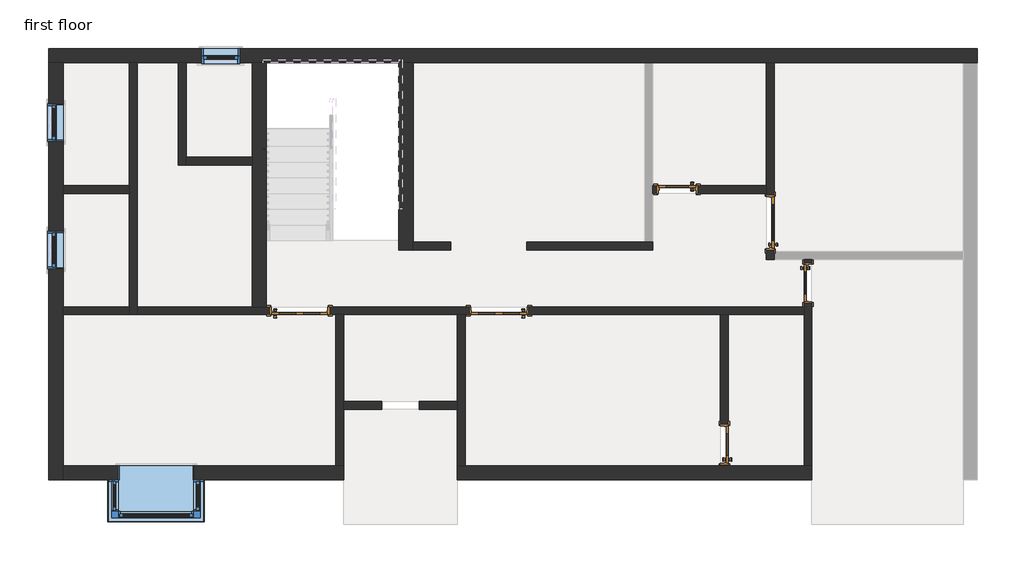
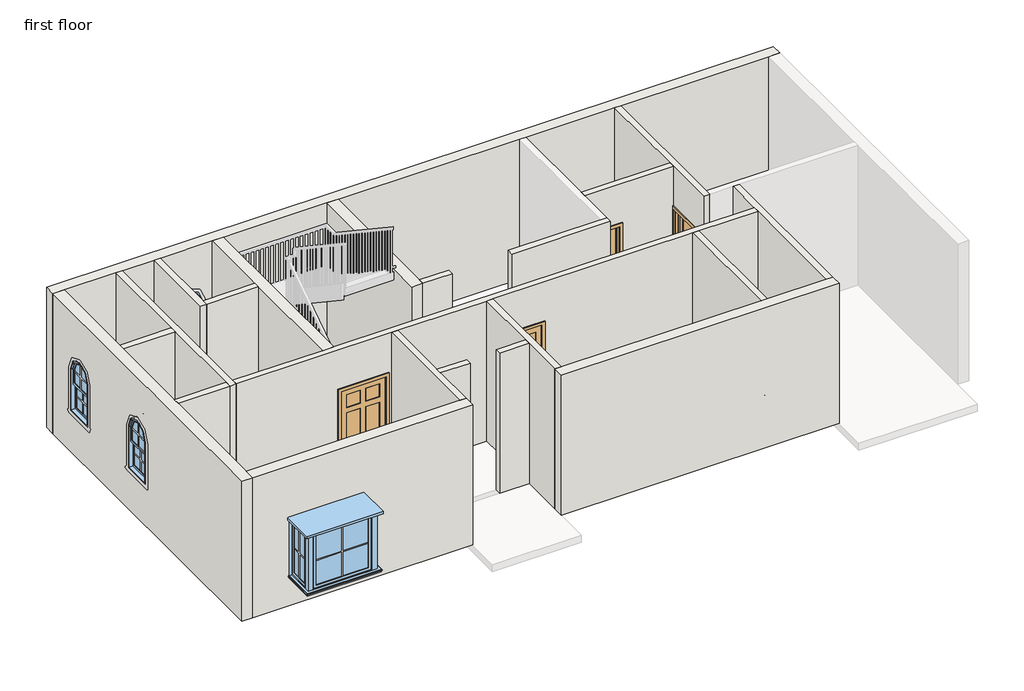
# One storey, part 1 of 3: 22 walls, 6 doors, 4 windows.
"""IFC4 building model written with IfcOpenShell, lengths in millimetres."""

from ifc_helpers import new_model, si_unit, frame, origin, place, context, project, spatial, polyline, circle_curve, outline, extrude, faceted_brep, transform, mapped, element, save
from ifc_brep_helpers import plane_surface, revolved_surface, advanced_brep
from components import door_e337afa5, door_6500584b, door_c610b25b, door_03e3dfb5, window_4fde904e, window_777a1d98

model = new_model("IFC4")

# Units and contexts
model_context = context("Model", 3, world=origin())
ifc_project = project(units=[si_unit("LENGTHUNIT", "METRE", prefix="MILLI")], contexts=[model_context])

# Site, building, storey
site = spatial("IfcSite", under=ifc_project)
building = spatial("IfcBuilding", under=site)
storey = spatial("IfcBuildingStorey", under=building, Name="first floor", Elevation=3352.8)

# Doors
placement = place(None, origin())
door_shape = door_e337afa5(model_context)
element("IfcDoor", 1, ObjectType="Door-Interior-Single-2_Panel-Wood : 24\" x 84\"", at=placement, inside=storey, context=model_context, shape_type="MappedRepresentation", body=[
    mapped(door_shape, transform((-2291.9922301, -6693.7302427, 3352.8), x_axis=(0.0, 1.0, 0.0), y_axis=(-1.0, 0.0, 0.0), z_axis=(0.0, 0.0, 1.0))),
])
element("IfcDoor", 2, ObjectType="Door-Interior-Single-2_Panel-Wood : 24\" x 84\"", at=placement, inside=storey, context=model_context, shape_type="MappedRepresentation", body=[
    mapped(door_shape, transform((-952.1422301, -4090.2302427, 3352.8), x_axis=(0.0, -1.0, 0.0), y_axis=(1.0, 0.0, 0.0), z_axis=(0.0, 0.0, 1.0))),
])
element("IfcDoor", 3, ObjectType="Door-Interior-Single-2_Panel-Wood : 24\" x 84\"", at=placement, inside=storey, context=model_context, shape_type="MappedRepresentation", body=[
    mapped(door_shape, transform((-3057.1672301, -2575.7552427, 3352.8), x_axis=(-1.0, 0.0, 0.0), y_axis=(0.0, -1.0, 0.0), z_axis=(0.0, 0.0, 1.0))),
])
door_2_shape = door_6500584b(model_context)
element("IfcDoor", 4, ObjectType="Door-Interior-Single-3_Panel_Vert-Wood : 33\" x 84\"", at=placement, inside=storey, context=model_context, shape_type="MappedRepresentation", body=[
    mapped(door_2_shape, transform((-1555.3922301, -3112.3302427, 3352.8), x_axis=(0.0, 1.0, 0.0), y_axis=(-1.0, 0.0, 0.0), z_axis=(0.0, 0.0, 1.0))),
])
door_3_shape = door_c610b25b(model_context)
element("IfcDoor", 5, ObjectType="Door-Interior-Single-6_Panel-Wood : 36\" x 84\"", at=placement, inside=storey, context=model_context, shape_type="MappedRepresentation", body=[
    mapped(door_3_shape, transform((-9140.4672301, -4537.9052427, 3352.8), x_axis=(1.0, 0.0, 0.0), y_axis=(0.0, 1.0, 0.0), z_axis=(0.0, 0.0, 1.0))),
])
door_4_shape = door_03e3dfb5(model_context)
element("IfcDoor", 6, ObjectType="Door-Interior-Single-6_Panel-Wood : 36\" x 84\"", at=placement, inside=storey, context=model_context, shape_type="MappedRepresentation", body=[
    mapped(door_4_shape, transform((-5927.3672301, -4537.9052427, 3352.8), x_axis=(-1.0, 0.0, 0.0), y_axis=(0.0, -1.0, 0.0), z_axis=(0.0, 0.0, 1.0))),
])

# Walls
element("IfcWall", 7, ObjectType="INNER WALL 5\"", at=placement, inside=storey, context=model_context, shape_type="SweptSolid", body=[
    extrude(outline(polyline([(-11883.6672301, -2642.4302427), (-12950.4672301, -2642.4302427), (-12950.4672301, -2515.4302427), (-11883.6672301, -2515.4302427), (-11883.6672301, -2642.4302427)])), frame((0.0, 0.0, 3352.8), z_axis=(0.0, 0.0, 1.0), x_axis=(1.0, 0.0, 0.0)), (0.0, 0.0, 1.0), 3048.0),
])
element("IfcWall", 8, ObjectType="INNER WALL 5\"", at=placement, inside=storey, context=model_context, shape_type="Brep", body=[
    faceted_brep([(-11883.6672301, -534.2302427, 3352.8), (-11883.6672301, -2515.4302427, 3352.8), (-11883.6672301, -2642.4302427, 3352.8), (-11883.6672301, -4471.2302427, 3352.8), (-11883.6672301, -4598.2302427, 3352.8), (-11883.6672301, -4598.2302427, 6400.8), (-11883.6672301, -4471.2302427, 6400.8), (-11883.6672301, -2642.4302427, 6400.8), (-11883.6672301, -2515.4302427, 6400.8), (-11883.6672301, -534.2302427, 6400.8), (-11756.6672301, -534.2302427, 3352.8), (-11756.6672301, -534.2302427, 6400.8), (-11756.6672301, -4471.2302427, 6400.8), (-11756.6672301, -4598.2302427, 6400.8), (-11756.6672301, -4598.2302427, 3352.8), (-11756.6672301, -4471.2302427, 3352.8)], [[[0, 1, 2, 3, 4, 5, 6, 7, 8, 9]], [[10, 11, 12, 13, 14, 15]], [[4, 3, 2, 1, 0, 10, 15, 14]], [[9, 8, 7, 6, 5, 13, 12, 11]], [[5, 4, 14, 13]], [[0, 9, 11, 10]]]),
])
element("IfcWall", 9, ObjectType="INNER WALL 5\"", at=placement, inside=storey, context=model_context, shape_type="SweptSolid", body=[
    extrude(outline(polyline([(-11883.6672301, -4598.2302427), (-12950.4672301, -4598.2302427), (-12950.4672301, -4471.2302427), (-11883.6672301, -4471.2302427), (-11883.6672301, -4598.2302427)])), frame((0.0, 0.0, 3352.8), z_axis=(0.0, 0.0, 1.0), x_axis=(1.0, 0.0, 0.0)), (0.0, 0.0, 1.0), 3048.0),
])
element("IfcWall", 10, ObjectType="INNER WALL 5\"", at=placement, inside=storey, context=model_context, shape_type="Brep", body=[
    faceted_brep([(-11096.2672301, -534.2302427, 3352.8), (-11096.2672301, -2185.2302427, 3352.8), (-11096.2672301, -2185.2302427, 6400.8), (-11096.2672301, -534.2302427, 6400.8), (-10969.2672301, -534.2302427, 3352.8), (-10969.2672301, -534.2302427, 6400.8), (-10969.2672301, -2058.2302427, 6400.8), (-10969.2672301, -2185.2302427, 6400.8), (-10969.2672301, -2185.2302427, 3352.8), (-10969.2672301, -2058.2302427, 3352.8)], [[[0, 1, 2, 3]], [[4, 5, 6, 7, 8, 9]], [[1, 0, 4, 9, 8]], [[3, 2, 7, 6, 5]], [[0, 3, 5, 4]], [[2, 1, 8, 7]]]),
])
element("IfcWall", 11, ObjectType="INNER WALL 5\"", at=placement, inside=storey, context=model_context, shape_type="SweptSolid", body=[
    extrude(outline(polyline([(-10969.2672301, -2058.2302427), (-9902.4672301, -2058.2302427), (-9902.4672301, -2185.2302427), (-10969.2672301, -2185.2302427), (-10969.2672301, -2058.2302427)])), frame((0.0, 0.0, 3352.8), z_axis=(0.0, 0.0, 1.0), x_axis=(1.0, 0.0, 0.0)), (0.0, 0.0, 1.0), 3048.0),
])
element("IfcWall", 12, ObjectType="INNER WALL 5\"", at=placement, inside=storey, context=model_context, shape_type="SweptSolid", body=[
    extrude(outline(polyline([(-6702.0672301, -3556.8302427), (-7311.6672301, -3556.8302427), (-7311.6672301, -3429.8302427), (-6702.0672301, -3429.8302427), (-6702.0672301, -3556.8302427)])), frame((0.0, 0.0, 3352.8), z_axis=(0.0, 0.0, 1.0), x_axis=(1.0, 0.0, 0.0)), (0.0, 0.0, 1.0), 3048.0),
])
element("IfcWall", 13, ObjectType="INNER WALL 5\"", at=placement, inside=storey, context=model_context, shape_type="Brep", body=[
    faceted_brep([(-5482.8672301, -3556.8302427, 3352.8), (-3450.8672301, -3556.8302427, 3352.8), (-3450.8672301, -3556.8302427, 6400.8), (-5482.8672301, -3556.8302427, 6400.8), (-5482.8672301, -3429.8302427, 3352.8), (-5482.8672301, -3429.8302427, 6400.8), (-3577.8672301, -3429.8302427, 6400.8), (-3450.8672301, -3429.8302427, 6400.8), (-3450.8672301, -3429.8302427, 3352.8), (-3577.8672301, -3429.8302427, 3352.8)], [[[0, 1, 2, 3]], [[4, 5, 6, 7, 8, 9]], [[1, 0, 4, 9, 8]], [[3, 2, 7, 6, 5]], [[0, 3, 5, 4]], [[2, 1, 8, 7]]]),
])
element("IfcWall", 14, ObjectType="INNER WALL 5\"", at=placement, inside=storey, context=model_context, shape_type="Brep", body=[
    faceted_brep([(-1622.0672301, -3709.2302427, 6400.8), (-1622.0672301, -2642.4302427, 6400.8), (-1622.0672301, -2515.4302427, 6400.8), (-1622.0672301, -534.2302427, 6400.8), (-1622.0672301, -534.2302427, 3352.8), (-1622.0672301, -2515.4302427, 3352.8), (-1622.0672301, -2642.4302427, 3352.8), (-1622.0672301, -2667.8302427, 3352.8), (-1622.0672301, -2667.8302427, 5511.8), (-1622.0672301, -3556.8302427, 5511.8), (-1622.0672301, -3556.8302427, 3352.8), (-1622.0672301, -3709.2302427, 3352.8), (-1495.0672301, -534.2302427, 6400.8), (-1495.0672301, -3582.2302427, 6400.8), (-1495.0672301, -3709.2302427, 6400.8), (-1495.0672301, -3709.2302427, 3352.8), (-1495.0672301, -3582.2302427, 3352.8), (-1495.0672301, -3556.8302427, 3352.8), (-1495.0672301, -3556.8302427, 5511.8), (-1495.0672301, -2667.8302427, 5511.8), (-1495.0672301, -2667.8302427, 3352.8), (-1495.0672301, -534.2302427, 3352.8)], [[[0, 1, 2, 3, 4, 5, 6, 7, 8, 9, 10, 11]], [[12, 13, 14, 15, 16, 17, 18, 19, 20, 21]], [[4, 21, 20, 7, 6, 5]], [[15, 11, 10, 17, 16]], [[3, 2, 1, 0, 14, 13, 12]], [[4, 3, 12, 21]], [[0, 11, 15, 14]], [[19, 8, 7, 20]], [[8, 19, 18, 9]], [[9, 18, 17, 10]]]),
])
element("IfcWall", 15, ObjectType="INNER WALL 5\"", at=placement, inside=storey, context=model_context, shape_type="SweptSolid", body=[
    extrude(outline(polyline([(6400.8, -1622.0672301), (6400.8, -3450.8672301), (3352.8, -3450.8672301), (3352.8, -3387.3672301), (5511.8, -3387.3672301), (5511.8, -2726.9672301), (3352.8, -2726.9672301), (3352.8, -1622.0672301), (6400.8, -1622.0672301)])), frame((0.0, -2642.4302427, 0.0), z_axis=(0.0, 1.0, 0.0), x_axis=(0.0, 0.0, 1.0)), (0.0, 0.0, 1.0), 127.0),
])
element("IfcWall", 16, ObjectType="INNER WALL 5\"", at=placement, inside=storey, context=model_context, shape_type="Brep", body=[
    faceted_brep([(-885.4672301, -3709.2302427, 6400.8), (-885.4672301, -7036.6302427, 6400.8), (-885.4672301, -7036.6302427, 3352.8), (-885.4672301, -4420.4302427, 3352.8), (-885.4672301, -4420.4302427, 5511.8), (-885.4672301, -3760.0302427, 5511.8), (-885.4672301, -3760.0302427, 3352.8), (-885.4672301, -3709.2302427, 3352.8), (-1012.4672301, -7036.6302427, 6400.8), (-1012.4672301, -4598.2302427, 6400.8), (-1012.4672301, -4471.2302427, 6400.8), (-1012.4672301, -3709.2302427, 6400.8), (-1012.4672301, -3709.2302427, 3352.8), (-1012.4672301, -3760.0302427, 3352.8), (-1012.4672301, -3760.0302427, 5511.8), (-1012.4672301, -4420.4302427, 5511.8), (-1012.4672301, -4420.4302427, 3352.8), (-1012.4672301, -4471.2302427, 3352.8), (-1012.4672301, -4598.2302427, 3352.8), (-1012.4672301, -7036.6302427, 3352.8)], [[[0, 1, 2, 3, 4, 5, 6, 7]], [[8, 9, 10, 11, 12, 13, 14, 15, 16, 17, 18, 19]], [[2, 19, 18, 17, 16, 3]], [[12, 7, 6, 13]], [[1, 0, 11, 10, 9, 8]], [[2, 1, 8, 19]], [[0, 7, 12, 11]], [[15, 4, 3, 16]], [[4, 15, 14, 5]], [[5, 14, 13, 6]]]),
])
element("IfcWall", 17, ObjectType="INNER WALL 5\"", at=placement, inside=storey, context=model_context, shape_type="Brep", body=[
    faceted_brep([(-11756.6672301, -4471.2302427, 6400.8), (-9902.4672301, -4471.2302427, 6400.8), (-9673.8672301, -4471.2302427, 6400.8), (-1012.4672301, -4471.2302427, 6400.8), (-1012.4672301, -4471.2302427, 3352.8), (-5444.7672301, -4471.2302427, 3352.8), (-5444.7672301, -4471.2302427, 5511.8), (-6409.9672301, -4471.2302427, 5511.8), (-6409.9672301, -4471.2302427, 3352.8), (-8657.8672301, -4471.2302427, 3352.8), (-8657.8672301, -4471.2302427, 5511.8), (-9623.0672301, -4471.2302427, 5511.8), (-9623.0672301, -4471.2302427, 3352.8), (-9673.8672301, -4471.2302427, 3352.8), (-9902.4672301, -4471.2302427, 3352.8), (-11756.6672301, -4471.2302427, 3352.8), (-1012.4672301, -4598.2302427, 6400.8), (-2231.6672301, -4598.2302427, 6400.8), (-2358.6672301, -4598.2302427, 6400.8), (-6473.4672301, -4598.2302427, 6400.8), (-6600.4672301, -4598.2302427, 6400.8), (-8429.2672301, -4598.2302427, 6400.8), (-8556.2672301, -4598.2302427, 6400.8), (-11756.6672301, -4598.2302427, 6400.8), (-11756.6672301, -4598.2302427, 3352.8), (-9623.0672301, -4598.2302427, 3352.8), (-9623.0672301, -4598.2302427, 5511.8), (-8657.8672301, -4598.2302427, 5511.8), (-8657.8672301, -4598.2302427, 3352.8), (-8556.2672301, -4598.2302427, 3352.8), (-8429.2672301, -4598.2302427, 3352.8), (-6600.4672301, -4598.2302427, 3352.8), (-6473.4672301, -4598.2302427, 3352.8), (-6409.9672301, -4598.2302427, 3352.8), (-6409.9672301, -4598.2302427, 5511.8), (-5444.7672301, -4598.2302427, 5511.8), (-5444.7672301, -4598.2302427, 3352.8), (-2358.6672301, -4598.2302427, 3352.8), (-2231.6672301, -4598.2302427, 3352.8), (-1012.4672301, -4598.2302427, 3352.8)], [[[0, 1, 2, 3, 4, 5, 6, 7, 8, 9, 10, 11, 12, 13, 14, 15]], [[16, 17, 18, 19, 20, 21, 22, 23, 24, 25, 26, 27, 28, 29, 30, 31, 32, 33, 34, 35, 36, 37, 38, 39]], [[4, 39, 38, 37, 36, 5]], [[24, 15, 14, 13, 12, 25]], [[28, 9, 8, 33, 32, 31, 30, 29]], [[3, 2, 1, 0, 23, 22, 21, 20, 19, 18, 17, 16]], [[4, 3, 16, 39]], [[0, 15, 24, 23]], [[27, 10, 9, 28]], [[10, 27, 26, 11]], [[11, 26, 25, 12]], [[7, 34, 33, 8]], [[34, 7, 6, 35]], [[35, 6, 5, 36]]]),
])
element("IfcWall", 18, ObjectType="INNER WALL 5\"", at=placement, inside=storey, context=model_context, shape_type="Brep", body=[
    faceted_brep([(-8556.2672301, -4598.2302427, 3352.8), (-8556.2672301, -7036.6302427, 3352.8), (-8556.2672301, -7036.6302427, 6400.8), (-8556.2672301, -4598.2302427, 6400.8), (-8429.2672301, -4598.2302427, 3352.8), (-8429.2672301, -4598.2302427, 6400.8), (-8429.2672301, -5995.2302427, 6400.8), (-8429.2672301, -6122.2302427, 6400.8), (-8429.2672301, -7036.6302427, 6400.8), (-8429.2672301, -7036.6302427, 3352.8), (-8429.2672301, -6122.2302427, 3352.8), (-8429.2672301, -5995.2302427, 3352.8)], [[[0, 1, 2, 3]], [[4, 5, 6, 7, 8, 9, 10, 11]], [[1, 0, 4, 11, 10, 9]], [[3, 2, 8, 7, 6, 5]], [[0, 3, 5, 4]], [[2, 1, 9, 8]]]),
])
element("IfcWall", 19, ObjectType="INNER WALL 5\"", at=placement, inside=storey, context=model_context, shape_type="SweptSolid", body=[
    extrude(outline(polyline([(-7819.6672301, -6122.2302427), (-8429.2672301, -6122.2302427), (-8429.2672301, -5995.2302427), (-7819.6672301, -5995.2302427), (-7819.6672301, -6122.2302427)])), frame((0.0, 0.0, 3352.8), z_axis=(0.0, 0.0, 1.0), x_axis=(1.0, 0.0, 0.0)), (0.0, 0.0, 1.0), 3048.0),
])
element("IfcWall", 20, ObjectType="INNER WALL 5\"", at=placement, inside=storey, context=model_context, shape_type="SweptSolid", body=[
    extrude(outline(polyline([(-6600.4672301, -6122.2302427), (-7210.0672301, -6122.2302427), (-7210.0672301, -5995.2302427), (-6600.4672301, -5995.2302427), (-6600.4672301, -6122.2302427)])), frame((0.0, 0.0, 3352.8), z_axis=(0.0, 0.0, 1.0), x_axis=(1.0, 0.0, 0.0)), (0.0, 0.0, 1.0), 3048.0),
])
element("IfcWall", 21, ObjectType="INNER WALL 5\"", at=placement, inside=storey, context=model_context, shape_type="Brep", body=[
    faceted_brep([(-6600.4672301, -4598.2302427, 3352.8), (-6600.4672301, -5995.2302427, 3352.8), (-6600.4672301, -6122.2302427, 3352.8), (-6600.4672301, -7036.6302427, 3352.8), (-6600.4672301, -7036.6302427, 6400.8), (-6600.4672301, -6122.2302427, 6400.8), (-6600.4672301, -5995.2302427, 6400.8), (-6600.4672301, -4598.2302427, 6400.8), (-6473.4672301, -4598.2302427, 3352.8), (-6473.4672301, -4598.2302427, 6400.8), (-6473.4672301, -7036.6302427, 6400.8), (-6473.4672301, -7036.6302427, 3352.8)], [[[0, 1, 2, 3, 4, 5, 6, 7]], [[8, 9, 10, 11]], [[3, 2, 1, 0, 8, 11]], [[7, 6, 5, 4, 10, 9]], [[4, 3, 11, 10]], [[0, 7, 9, 8]]]),
])
element("IfcWall", 22, ObjectType="INNER WALL 5\"", at=placement, inside=storey, context=model_context, shape_type="SweptSolid", body=[
    extrude(outline(polyline([(-7036.6302427, 6400.8), (-4598.2302427, 6400.8), (-4598.2302427, 3352.8), (-6363.5302427, 3352.8), (-6363.5302427, 5511.8), (-7023.9302427, 5511.8), (-7023.9302427, 3352.8), (-7036.6302427, 3352.8), (-7036.6302427, 6400.8)])), frame((-2358.6672301, 0.0, 0.0), z_axis=(1.0, 0.0, 0.0), x_axis=(0.0, 1.0, 0.0)), (0.0, 0.0, 1.0), 127.0),
])
element("IfcWall", 23, ObjectType="OUTER WALL 9\"", at=placement, inside=storey, context=model_context, shape_type="AdvancedBrep", body=[
    advanced_brep(
    [(-13179.0672301, -534.2302427, 3352.8), (-12950.4672301, -534.2302427, 3352.8), (-11883.6672301, -534.2302427, 3352.8), (-11756.6672301, -534.2302427, 3352.8), (-11096.2672301, -534.2302427, 3352.8), (-10969.2672301, -534.2302427, 3352.8), (-9902.4672301, -534.2302427, 3352.8), (-9673.8672301, -534.2302427, 3352.8), (-7540.2672301, -534.2302427, 3352.8), (-7311.6672301, -534.2302427, 3352.8), (-3577.8672301, -534.2302427, 3352.8), (-3450.8672301, -534.2302427, 3352.8), (-1622.0672301, -534.2302427, 3352.8), (-1495.0672301, -534.2302427, 3352.8), (1552.9327699, -534.2302427, 3352.8), (1781.5327699, -534.2302427, 3352.8), (1781.5327699, -534.2302427, 6400.8), (1552.9327699, -534.2302427, 6400.8), (-1495.0672301, -534.2302427, 6400.8), (-1622.0672301, -534.2302427, 6400.8), (-3450.8672301, -534.2302427, 6400.8), (-3577.8672301, -534.2302427, 6400.8), (-7311.6672301, -534.2302427, 6400.8), (-7540.2672301, -534.2302427, 6400.8), (-9673.8672301, -534.2302427, 6400.8), (-9902.4672301, -534.2302427, 6400.8), (-10969.2672301, -534.2302427, 6400.8), (-11096.2672301, -534.2302427, 6400.8), (-11756.6672301, -534.2302427, 6400.8), (-11883.6672301, -534.2302427, 6400.8), (-12950.4672301, -534.2302427, 6400.8), (-13179.0672301, -534.2302427, 6400.8), (-10715.2672301, -534.2302427, 5181.6), (-10105.6672301, -534.2302427, 5181.6), (-10105.6672301, -534.2302427, 4267.2), (-10715.2672301, -534.2302427, 4267.2), (-13179.0672301, -305.6302427, 3352.8), (-13179.0672301, -305.6302427, 6400.8), (1781.5327699, -305.6302427, 6400.8), (1781.5327699, -305.6302427, 3352.8), (-10715.2672301, -305.6302427, 5181.6), (-10715.2672301, -305.6302427, 4267.2), (-10105.6672301, -305.6302427, 4267.2), (-10105.6672301, -305.6302427, 5181.6)],
    [
        (0, 1),
        (1, 2),
        (2, 3),
        (3, 4),
        (4, 5),
        (5, 6),
        (6, 7),
        (7, 8),
        (8, 9),
        (9, 10),
        (10, 11),
        (11, 12),
        (12, 13),
        (13, 14),
        (14, 15),
        (15, 16),
        (16, 17),
        (17, 18),
        (18, 19),
        (19, 20),
        (20, 21),
        (21, 22),
        (22, 23),
        (23, 24),
        (24, 25),
        (25, 26),
        (26, 27),
        (27, 28),
        (28, 29),
        (29, 30),
        (30, 31),
        (31, 0),
        (32, 33, circle_curve(frame((-10410.4672301, -534.2302427, 5181.6), z_axis=(0.0, 1.0, 0.0), x_axis=(-1.0, 0.0, 0.0)), 304.8)),
        (33, 34),
        (34, 35),
        (35, 32),
        (36, 37),
        (37, 38),
        (38, 39),
        (39, 36),
        (40, 41),
        (41, 42),
        (42, 43),
        (43, 40, circle_curve(frame((-10410.4672301, -305.6302427, 5181.6), z_axis=(0.0, -1.0, 0.0), x_axis=(-1.0, 0.0, 0.0)), 304.8)),
        (0, 36),
        (39, 15),
        (16, 38),
        (37, 31),
        (32, 40),
        (43, 33),
        (42, 34),
        (41, 35),
    ],
    [
        plane_surface(frame((-13170.1356678, -534.2302427, 3352.8), z_axis=(0.0, -1.0, 0.0), x_axis=(1.0, 0.0, 0.0))),
        plane_surface(frame((-13170.1356678, -305.6302427, 3352.8), z_axis=(0.0, 1.0, 0.0), x_axis=(-1.0, 0.0, 0.0))),
        plane_surface(frame((-13064.7672301, -534.2302427, 3352.8), z_axis=(0.0, 0.0, -1.0), x_axis=(0.0, 1.0, 0.0))),
        plane_surface(frame((1667.2327699, -534.2302427, 6400.8), z_axis=(0.0, 0.0, 1.0), x_axis=(0.0, 1.0, 0.0))),
        plane_surface(frame((-13179.0672301, -534.2302427, 3352.8), z_axis=(-1.0, 0.0, 0.0), x_axis=(0.0, -1.0, 0.0))),
        plane_surface(frame((1781.5327699, -7258.6414899, 3352.8), z_axis=(1.0, 0.0, 0.0), x_axis=(0.0, 1.0, 0.0))),
        revolved_surface(polyline([(-10715.267230099998, -305.6302427, 5181.6), (-10715.267230099998, -534.2302427, 5181.6)]), (-10410.4672301, -305.6302427, 5181.6), (0.0, 1.0, 0.0)),
        plane_surface(frame((-10105.6672301, -534.2302427, 5181.6), z_axis=(-1.0, 0.0, 0.0), x_axis=(0.0, 1.0, 0.0))),
        plane_surface(frame((-10105.6672301, -534.2302427, 4267.2), z_axis=(0.0, 0.0, 1.0), x_axis=(0.0, 1.0, 0.0))),
        plane_surface(frame((-10715.2672301, -534.2302427, 4267.2), z_axis=(1.0, 0.0, 0.0), x_axis=(0.0, 1.0, 0.0))),
    ],
    [
        (0, [[1, 2, 3, 4, 5, 6, 7, 8, 9, 10, 11, 12, 13, 14, 15, 16, 17, 18, 19, 20, 21, 22, 23, 24, 25, 26, 27, 28, 29, 30, 31, 32], [33, 34, 35, 36]]),
        (1, [[37, 38, 39, 40], [41, 42, 43, 44]]),
        (2, [[-15, -14, -13, -12, -11, -10, -9, -8, -7, -6, -5, -4, -3, -2, -1, 45, -40, 46]]),
        (3, [[-31, -30, -29, -28, -27, -26, -25, -24, -23, -22, -21, -20, -19, -18, -17, 47, -38, 48]]),
        (4, [[-32, -48, -37, -45]]),
        (5, [[-16, -46, -39, -47]]),
        (6, [[-33, 49, -44, 50]]),
        (7, [[-34, -50, -43, 51]]),
        (8, [[-35, -51, -42, 52]]),
        (9, [[-36, -52, -41, -49]]),
    ],
),
])
element("IfcWall", 24, ObjectType="OUTER WALL 9\"", at=placement, inside=storey, context=model_context, shape_type="AdvancedBrep", body=[
    advanced_brep(
    [(-13179.0672301, -534.2302427, 3352.8), (-13179.0672301, -7265.2302427, 3352.8), (-13179.0672301, -7265.2302427, 6400.8), (-13179.0672301, -534.2302427, 6400.8), (-13179.0672301, -1194.6302427, 5181.6), (-13179.0672301, -1804.2302427, 5181.6), (-13179.0672301, -1804.2302427, 4267.2), (-13179.0672301, -1194.6302427, 4267.2), (-13179.0672301, -3252.0302427, 5181.6), (-13179.0672301, -3861.6302427, 5181.6), (-13179.0672301, -3861.6302427, 4267.2), (-13179.0672301, -3252.0302427, 4267.2), (-12950.4672301, -534.2302427, 3352.8), (-12950.4672301, -534.2302427, 6400.8), (-12950.4672301, -2515.4302427, 6400.8), (-12950.4672301, -2642.4302427, 6400.8), (-12950.4672301, -4471.2302427, 6400.8), (-12950.4672301, -4598.2302427, 6400.8), (-12950.4672301, -7036.6302427, 6400.8), (-12950.4672301, -7265.2302427, 6400.8), (-12950.4672301, -7265.2302427, 3352.8), (-12950.4672301, -7036.6302427, 3352.8), (-12950.4672301, -4598.2302427, 3352.8), (-12950.4672301, -4471.2302427, 3352.8), (-12950.4672301, -2642.4302427, 3352.8), (-12950.4672301, -2515.4302427, 3352.8), (-12950.4672301, -1194.6302427, 5181.6), (-12950.4672301, -1194.6302427, 4267.2), (-12950.4672301, -1804.2302427, 4267.2), (-12950.4672301, -1804.2302427, 5181.6), (-12950.4672301, -3252.0302427, 5181.6), (-12950.4672301, -3252.0302427, 4267.2), (-12950.4672301, -3861.6302427, 4267.2), (-12950.4672301, -3861.6302427, 5181.6)],
    [
        (0, 1),
        (1, 2),
        (2, 3),
        (3, 0),
        (4, 5, circle_curve(frame((-13179.0672301, -1499.4302427, 5181.6), z_axis=(1.0, 0.0, 0.0), x_axis=(0.0, 1.0, 0.0)), 304.8)),
        (5, 6),
        (6, 7),
        (7, 4),
        (8, 9, circle_curve(frame((-13179.0672301, -3556.8302427, 5181.6), z_axis=(1.0, 0.0, 0.0), x_axis=(0.0, 1.0, 0.0)), 304.8)),
        (9, 10),
        (10, 11),
        (11, 8),
        (12, 13),
        (13, 14),
        (14, 15),
        (15, 16),
        (16, 17),
        (17, 18),
        (18, 19),
        (19, 20),
        (20, 21),
        (21, 22),
        (22, 23),
        (23, 24),
        (24, 25),
        (25, 12),
        (26, 27),
        (27, 28),
        (28, 29),
        (29, 26, circle_curve(frame((-12950.4672301, -1499.4302427, 5181.6), z_axis=(-1.0, 0.0, 0.0), x_axis=(0.0, 1.0, 0.0)), 304.8)),
        (30, 31),
        (31, 32),
        (32, 33),
        (33, 30, circle_curve(frame((-12950.4672301, -3556.8302427, 5181.6), z_axis=(-1.0, 0.0, 0.0), x_axis=(0.0, 1.0, 0.0)), 304.8)),
        (0, 12),
        (20, 1),
        (2, 19),
        (13, 3),
        (4, 26),
        (29, 5),
        (28, 6),
        (27, 7),
        (8, 30),
        (33, 9),
        (32, 10),
        (31, 11),
    ],
    [
        plane_surface(frame((-13179.0672301, -534.2302427, 3352.8), z_axis=(-1.0, 0.0, 0.0), x_axis=(0.0, -1.0, 0.0))),
        plane_surface(frame((-12950.4672301, -534.2302427, 3352.8), z_axis=(1.0, 0.0, 0.0), x_axis=(0.0, 1.0, 0.0))),
        plane_surface(frame((-13179.0672301, -419.9302427, 3352.8), z_axis=(0.0, 0.0, -1.0), x_axis=(1.0, 0.0, 0.0))),
        plane_surface(frame((-13179.0672301, -7150.9302427, 6400.8), z_axis=(0.0, 0.0, 1.0), x_axis=(1.0, 0.0, 0.0))),
        plane_surface(frame((-13170.1356678, -534.2302427, 3352.8), z_axis=(0.0, 1.0, 0.0), x_axis=(1.0, 0.0, 0.0))),
        plane_surface(frame((-13179.0672301, -7265.2302427, 3352.8), z_axis=(0.0, -1.0, 0.0), x_axis=(1.0, 0.0, 0.0))),
        revolved_surface(polyline([(-12950.4672301, -1194.6302427, 5181.6), (-13179.0672301, -1194.6302427, 5181.6)]), (-12950.4672301, -1499.4302427, 5181.6), (1.0, 0.0, 0.0)),
        plane_surface(frame((-13179.0672301, -1804.2302427, 5181.6), z_axis=(0.0, 1.0, 0.0), x_axis=(1.0, 0.0, 0.0))),
        plane_surface(frame((-13179.0672301, -1804.2302427, 4267.2), z_axis=(0.0, 0.0, 1.0), x_axis=(1.0, 0.0, 0.0))),
        plane_surface(frame((-13179.0672301, -1194.6302427, 4267.2), z_axis=(0.0, -1.0, 0.0), x_axis=(1.0, 0.0, 0.0))),
        revolved_surface(polyline([(-12950.4672301, -3252.0302426999997, 5181.6), (-13179.0672301, -3252.0302426999997, 5181.6)]), (-12950.4672301, -3556.8302427, 5181.6), (1.0, 0.0, 0.0)),
        plane_surface(frame((-13179.0672301, -3861.6302427, 5181.6), z_axis=(0.0, 1.0, 0.0), x_axis=(1.0, 0.0, 0.0))),
        plane_surface(frame((-13179.0672301, -3861.6302427, 4267.2), z_axis=(0.0, 0.0, 1.0), x_axis=(1.0, 0.0, 0.0))),
        plane_surface(frame((-13179.0672301, -3252.0302427, 4267.2), z_axis=(0.0, -1.0, 0.0), x_axis=(1.0, 0.0, 0.0))),
    ],
    [
        (0, [[1, 2, 3, 4], [5, 6, 7, 8], [9, 10, 11, 12]]),
        (1, [[13, 14, 15, 16, 17, 18, 19, 20, 21, 22, 23, 24, 25, 26], [27, 28, 29, 30], [31, 32, 33, 34]]),
        (2, [[-1, 35, -26, -25, -24, -23, -22, -21, 36]]),
        (3, [[-3, 37, -19, -18, -17, -16, -15, -14, 38]]),
        (4, [[-4, -38, -13, -35]]),
        (5, [[-2, -36, -20, -37]]),
        (6, [[-5, 39, -30, 40]]),
        (7, [[-6, -40, -29, 41]]),
        (8, [[-7, -41, -28, 42]]),
        (9, [[-8, -42, -27, -39]]),
        (10, [[-9, 43, -34, 44]]),
        (11, [[-10, -44, -33, 45]]),
        (12, [[-11, -45, -32, 46]]),
        (13, [[-12, -46, -31, -43]]),
    ],
),
])
element("IfcWall", 25, ObjectType="OUTER WALL 9\"", at=placement, inside=storey, context=model_context, shape_type="Brep", body=[
    faceted_brep([(-12950.4672301, -7265.2302427, 3352.8), (-8429.2672301, -7265.2302427, 3352.8), (-8429.2672301, -7265.2302427, 6400.8), (-12950.4672301, -7265.2302427, 6400.8), (-12061.4672301, -7265.2302427, 5232.4), (-10842.2672301, -7265.2302427, 5232.4), (-10842.2672301, -7265.2302427, 3962.4), (-12061.4672301, -7265.2302427, 3962.4), (-12950.4672301, -7036.6302427, 3352.8), (-12950.4672301, -7036.6302427, 6400.8), (-8556.2672301, -7036.6302427, 6400.8), (-8429.2672301, -7036.6302427, 6400.8), (-8429.2672301, -7036.6302427, 3352.8), (-8556.2672301, -7036.6302427, 3352.8), (-12061.4672301, -7036.6302427, 5232.4), (-12061.4672301, -7036.6302427, 3962.4), (-10842.2672301, -7036.6302427, 3962.4), (-10842.2672301, -7036.6302427, 5232.4)], [[[0, 1, 2, 3], [4, 5, 6, 7]], [[8, 9, 10, 11, 12, 13], [14, 15, 16, 17]], [[1, 0, 8, 13, 12]], [[3, 2, 11, 10, 9]], [[0, 3, 9, 8]], [[15, 14, 4, 7]], [[16, 15, 7, 6]], [[17, 16, 6, 5]], [[14, 17, 5, 4]], [[2, 1, 12, 11]]]),
])
element("IfcWall", 26, ObjectType="OUTER WALL 9\"", at=placement, inside=storey, context=model_context, shape_type="Brep", body=[
    faceted_brep([(-7540.2672301, -534.2302427, 3352.8), (-7540.2672301, -3556.8302427, 3352.8), (-7540.2672301, -3556.8302427, 6400.8), (-7540.2672301, -534.2302427, 6400.8), (-7311.6672301, -534.2302427, 3352.8), (-7311.6672301, -534.2302427, 6400.8), (-7311.6672301, -3429.8302427, 6400.8), (-7311.6672301, -3556.8302427, 6400.8), (-7311.6672301, -3556.8302427, 3352.8), (-7311.6672301, -3429.8302427, 3352.8)], [[[0, 1, 2, 3]], [[4, 5, 6, 7, 8, 9]], [[1, 0, 4, 9, 8]], [[3, 2, 7, 6, 5]], [[0, 3, 5, 4]], [[2, 1, 8, 7]]]),
])
element("IfcWall", 27, ObjectType="OUTER WALL 9\"", at=placement, inside=storey, context=model_context, shape_type="Brep", body=[
    faceted_brep([(-9902.4672301, -534.2302427, 3352.8), (-9902.4672301, -2058.2302427, 3352.8), (-9902.4672301, -2185.2302427, 3352.8), (-9902.4672301, -4471.2302427, 3352.8), (-9902.4672301, -4471.2302427, 6400.8), (-9902.4672301, -2185.2302427, 6400.8), (-9902.4672301, -2058.2302427, 6400.8), (-9902.4672301, -534.2302427, 6400.8), (-9673.8672301, -534.2302427, 3352.8), (-9673.8672301, -534.2302427, 6400.8), (-9673.8672301, -4471.2302427, 6400.8), (-9673.8672301, -4471.2302427, 3352.8)], [[[0, 1, 2, 3, 4, 5, 6, 7]], [[8, 9, 10, 11]], [[3, 2, 1, 0, 8, 11]], [[7, 6, 5, 4, 10, 9]], [[0, 7, 9, 8]], [[4, 3, 11, 10]]]),
])
element("IfcWall", 28, ObjectType="OUTER WALL 9\"", at=placement, inside=storey, context=model_context, shape_type="Brep", body=[
    faceted_brep([(-6600.4672301, -7265.2302427, 3352.8), (-885.4672301, -7265.2302427, 3352.8), (-885.4672301, -7265.2302427, 6400.8), (-6600.4672301, -7265.2302427, 6400.8), (-6600.4672301, -7036.6302427, 3352.8), (-6600.4672301, -7036.6302427, 6400.8), (-6473.4672301, -7036.6302427, 6400.8), (-2358.6672301, -7036.6302427, 6400.8), (-2231.6672301, -7036.6302427, 6400.8), (-1012.4672301, -7036.6302427, 6400.8), (-885.4672301, -7036.6302427, 6400.8), (-885.4672301, -7036.6302427, 3352.8), (-1012.4672301, -7036.6302427, 3352.8), (-2231.6672301, -7036.6302427, 3352.8), (-2358.6672301, -7036.6302427, 3352.8), (-6473.4672301, -7036.6302427, 3352.8)], [[[0, 1, 2, 3]], [[4, 5, 6, 7, 8, 9, 10, 11, 12, 13, 14, 15]], [[1, 0, 4, 15, 14, 13, 12, 11]], [[3, 2, 10, 9, 8, 7, 6, 5]], [[2, 1, 11, 10]], [[0, 3, 5, 4]]]),
])

# Windows
window_shape = window_4fde904e(model_context)
element("IfcWindow", 29, ObjectType="Window-Bay-Casement-Box-90_Degree_Angle-Center_Fixed : 48\" x 48\" x 24\" 2", at=placement, inside=storey, context=model_context, shape_type="MappedRepresentation", body=[
    mapped(window_shape, transform((-11451.8672301, -7150.9302427, 3352.8), x_axis=(-1.0, 0.0, 0.0), y_axis=(0.0, -1.0, 0.0), z_axis=(0.0, 0.0, 1.0))),
])
window_2_shape = window_777a1d98(model_context)
element("IfcWindow", 30, ObjectType="Window-Double-Hung-Arch-Head : 24\" x 48\"", at=placement, inside=storey, context=model_context, shape_type="MappedRepresentation", body=[
    mapped(window_2_shape, transform((-13064.7672301, -1499.4302427, 3352.8), x_axis=(0.0, 1.0, 0.0), y_axis=(-1.0, 0.0, 0.0), z_axis=(0.0, 0.0, 1.0))),
])
element("IfcWindow", 31, ObjectType="Window-Double-Hung-Arch-Head : 24\" x 48\"", at=placement, inside=storey, context=model_context, shape_type="MappedRepresentation", body=[
    mapped(window_2_shape, transform((-13064.7672301, -3556.8302427, 3352.8), x_axis=(0.0, 1.0, 0.0), y_axis=(-1.0, 0.0, 0.0), z_axis=(0.0, 0.0, 1.0))),
])
element("IfcWindow", 32, ObjectType="Window-Double-Hung-Arch-Head : 24\" x 48\"", at=placement, inside=storey, context=model_context, shape_type="MappedRepresentation", body=[
    mapped(window_2_shape, transform((-10410.4672301, -419.9302427, 3352.8), x_axis=(-1.0, 0.0, 0.0), y_axis=(0.0, -1.0, 0.0), z_axis=(0.0, 0.0, 1.0))),
])

save(model, "model.ifc")

# Revit data of these elements
# Type "Door-Interior-Single-2_Panel-Wood : 24\" x 84\""
#   Type Mark = "10"
#   Assembly Code = "C1020300"
#   Analytic Construction = "Wooden"
#   Top Rail = 0' - 4 11/16"
#   Thickness = 0' - 1 3/8"
#   Thermal Resistance (R) = 2.5876 (h·ft²·°F)/BTU
#   Swing Angle [instance default] = 90.00°
#   Stiles = 0' - 4 3/4"
#   Rough Width = 2' - 2"
#   Rough Height = 7' - 1"
#   Lock Rail = 0' - 7 1/2"
#   Height = 7' - 0"
#   Width = 2' - 0"
#   Heat Transfer Coefficient (U) = 0.3865 BTU/(h·ft²·°F)
#   Bottom Rail = 0' - 9 1/8"
#   Trim Material = Cherry
#   Panel Material = Cherry
#   Frame Material = Cherry
#   Door Handle Material = Aluminum
#   Visual Light Transmittance = 0
#   Solar Heat Gain Coefficient = 0
#   Wall Closure = (empty or 0)
#   Function = (empty or 0)
# Type "Door-Interior-Single-3_Panel_Vert-Wood : 33\" x 84\""
#   Type Mark = "11"
#   Assembly Code = "C1020300"
#   Analytic Construction = "Wooden"
#   Top Rail = 0' - 4 11/16"
#   Thickness = 0' - 1 3/8"
#   Thermal Resistance (R) = 2.5876 (h·ft²·°F)/BTU
#   Swing Angle [instance default] = 90.00°
#   Stiles = 0' - 4 3/4"
#   Rough Width = 2' - 11"
#   Rough Height = 7' - 1"
#   Intermediate Rail = 0' - 4 1/2"
#   Height = 7' - 0"
#   Width = 2' - 9"
#   Heat Transfer Coefficient (U) = 0.3865 BTU/(h·ft²·°F)
#   Bottom Rail = 0' - 9 1/8"
#   Trim Material = Cherry
#   Panel Material = Cherry
#   Frame Material = Cherry
#   Door Handle Material = Aluminum
#   Visual Light Transmittance = 0
#   Solar Heat Gain Coefficient = 0
#   Wall Closure = (empty or 0)
#   Function = (empty or 0)
# Type "Door-Interior-Single-6_Panel-Wood : 36\" x 84\""
#   Type Mark = "12"
#   Assembly Code = "C1020300"
#   Analytic Construction = "Wooden"
#   Top Rail = 0' - 4 11/16"
#   Top Panel = 0' - 11"
#   Thickness = 0' - 1 3/8"
#   Thermal Resistance (R) = 2.5876 (h·ft²·°F)/BTU
#   Swing Angle [instance default] = 90.00°
#   Stiles = 0' - 4 3/4"
#   Rough Width = 3' - 2"
#   Rough Height = 7' - 1"
#   Mullion = 0' - 4 1/2"
#   Lock Rail = 0' - 7 1/2"
#   Intermediate Rail = 0' - 4 1/2"
#   Height = 7' - 0"
#   Width = 3' - 0"
#   Heat Transfer Coefficient (U) = 0.3865 BTU/(h·ft²·°F)
#   Bottom Rail = 0' - 9 1/8"
#   Trim Material = Cherry
#   Panel Material = Cherry
#   Frame Material = Cherry
#   Door Handle Material = Aluminum
#   Visual Light Transmittance = 0
#   Solar Heat Gain Coefficient = 0
#   Wall Closure = (empty or 0)
#   Function = (empty or 0)
# Type "INNER WALL 5\""
#   Assembly Code = "B2010"
#   Layers, outside or top first: 0' - 5" "WARM BEIGE COLOUR" (function 1)
# Type "OUTER WALL 9\""
#   Assembly Code = "B2010"
#   Layers, outside or top first: 0' - 9" "WARM BEIGE COLOUR" (function 1)
# Type "Window-Bay-Casement-Box-90_Degree_Angle-Center_Fixed : 48\" x 48\" x 24\" 2"
#   Type Mark = "22"
#   Fire Rating = "0.5h"
#   Assembly Code = "B2020100"
#   Analytic Construction = "1/8 in Pilkington single glazing"
#   Width = 4' - 0"
#   Wall Thickness [instance default] = 0' - 6"
#   Visual Light Transmittance = 0.9
#   Trim Width = 4' - 8"
#   Trim Height = 4' - 0"
#   Thermal Resistance (R) = 1.5394 (h·ft²·°F)/BTU
#   Solar Heat Gain Coefficient = 0.86
#   Rough Width = 4' - 0 1/2"
#   Rough Height = 4' - 0 1/2"
#   Height 1 = 4' - 2"
#   Height = 4' - 0"
#   Heat Transfer Coefficient (U) = 0.6496 BTU/(h·ft²·°F)
#   Depth = 2' - 0"
#   Default Sill Height = 2' - 0"
#   Side Muntin Visibility = yes
#   Center Muntin Visibility = yes
#   Interior Trim Visibility [instance default] = yes
#   Exterior Trim Visibility [instance default] = yes
#   Side Muntin Pattern = Muntin Pattern_2x2 : Muntin Pattern_2x2
#   Center Muntin Pattern = Muntin Pattern_2x2 : Muntin Pattern_2x2
#   Interior Trim Material = Wood - Stained
#   Exterior Trim Material = Clad - White
#   Exterior Trim = element 393412
#   Interior Trim = Trim-Window-Interior-Flat : Picture Frame
#   Interior Frame Material = Wood - Stained
#   Glass Panel Material = Glass
#   Exterior Frame Material = Clad - White
#   Wall Closure = (empty or 0)
# Type "Window-Double-Hung-Arch-Head : 24\" x 48\""
#   Type Mark = "19"
#   Fire Rating = "0.5h"
#   Construction Type Id = "DG-DR"
#   Assembly Code = "B2020100"
#   Analytic Construction = "Double glazing - domestic"
#   Wall Thickness [instance default] = 0' - 6"
#   Window Inset [instance default] = 0' - 0"
#   Visual Light Transmittance = 0.81
#   Thermal Resistance (R) = 1.8146 (h·ft²·°F)/BTU
#   Solar Heat Gain Coefficient = 0.76
#   Muntin Width = 1' - 6"
#   Muntin Height = 1' - 8 1/8"
#   Interior Wall Closure [instance default] = 0' - 1 1/2"
#   Rough Width = 2' - 0 1/2"
#   Rough Height = 4' - 0 1/2"
#   Half Width = 1' - 0"
#   Frame Extension [instance default] = 0' - 1 1/4"
#   Exterior Wall Closure [instance default] = 0' - 0 1/2"
#   Extension Jamb [instance default] = 0' - 1 1/2"
#   Heat Transfer Coefficient (U) = 0.5511 BTU/(h·ft²·°F)
#   Height = 4' - 0"
#   Width = 2' - 0"
#   Top Muntin Visibility = yes
#   Indicator Visibility [instance default] = yes
#   Extension Jamb Visibility [instance default] = yes
#   Interior Trim Visibility [instance default] = yes
#   Exterior Trim Visibility [instance default] = yes
#   Define Thermal Properties by = 1
#   Bottom Muntin Visibility = yes
#   Muntin Pattern = Muntin Pattern_2x2 : Muntin Pattern_2x2
#   Interior Trim Material = Wood - Stained
#   Interior Trim = Trim-Window-Interior-Arch-Hung : Picture Frame
#   Exterior Trim Material = Clad - White
#   Exterior Trim = Trim-Window-Exterior-Arch-Hung : with Sill
#   Glass Panel Material = Glass
#   Exterior Frame Material = Clad - White
#   Interior Frame Material = Wood - Stained
#   Wall Closure = (empty or 0)
# Elements 1, 2, 3 (IfcDoor, "Door-Interior-Single-2_Panel-Wood : 24\" x 84\"")
#   Swing Angle = 90.00°
#   Phase Created = New Construction
#   Materials on its faces: "Cherry", "Aluminum"
# Element 4 (IfcDoor, "Door-Interior-Single-3_Panel_Vert-Wood : 33\" x 84\"")
#   Swing Angle = 90.00°
#   Phase Created = New Construction
#   Materials on its faces: "Cherry", "Aluminum"
# Elements 5, 6 (IfcDoor, "Door-Interior-Single-6_Panel-Wood : 36\" x 84\"")
#   Swing Angle = 90.00°
#   Phase Created = New Construction
#   Materials on its faces: "Cherry", "Aluminum"
# Elements 7, 8, 9, 10, 11, 12, 13, 14, 15, 16, 17, 18, 19, 20, 21, 22 (IfcWall, "INNER WALL 5\"")
#   Top Offset = 0' - 0"
#   Base Offset = 0' - 0"
#   wall height = 10' - 0"
#   Phase Created = New Construction
#   Base Constraint = first floor
#   Top Constraint = TOP OF THE BUILDING
#   Materials on its faces: "WARM BEIGE COLOUR"
# Elements 23, 24, 25, 26, 27, 28 (IfcWall, "OUTER WALL 9\"")
#   Top Offset = 0' - 0"
#   Base Offset = 0' - 0"
#   wall height = 10' - 0"
#   Phase Created = New Construction
#   Base Constraint = first floor
#   Top Constraint = TOP OF THE BUILDING
#   Materials on its faces: "WARM BEIGE COLOUR"
# Element 29 (IfcWindow, "Window-Bay-Casement-Box-90_Degree_Angle-Center_Fixed : 48\" x 48\" x 24\" 2")
#   Mark = "8"
#   Interior Trim Visibility = yes
#   Exterior Trim Visibility = yes
#   Phase Created = New Construction
#   Materials on its faces: "Clad - White", "Wood - Stained", "Glass"
# Element 30 (IfcWindow, "Window-Double-Hung-Arch-Head : 24\" x 48\"")
#   Mark = "9"
#   Window Inset = 0' - 0"
#   Interior Wall Closure = 0' - 1 1/2"
#   Frame Extension = 0' - 1 1/4"
#   Exterior Wall Closure = 0' - 0 1/2"
#   Interior Trim Visibility = yes
#   Indicator Visibility = yes
#   Exterior Trim Visibility = yes
#   Phase Created = New Construction
#   Materials on its faces: "Wood - Stained", "Glass", "Clad - White"
# Element 31 (IfcWindow, "Window-Double-Hung-Arch-Head : 24\" x 48\"")
#   Mark = "10"
#   Window Inset = 0' - 0"
#   Interior Wall Closure = 0' - 1 1/2"
#   Frame Extension = 0' - 1 1/4"
#   Exterior Wall Closure = 0' - 0 1/2"
#   Interior Trim Visibility = yes
#   Indicator Visibility = yes
#   Exterior Trim Visibility = yes
#   Phase Created = New Construction
#   Materials on its faces: "Wood - Stained", "Glass", "Clad - White"
# Element 32 (IfcWindow, "Window-Double-Hung-Arch-Head : 24\" x 48\"")
#   Mark = "11"
#   Window Inset = 0' - 0"
#   Interior Wall Closure = 0' - 1 1/2"
#   Frame Extension = 0' - 1 1/4"
#   Exterior Wall Closure = 0' - 0 1/2"
#   Interior Trim Visibility = yes
#   Indicator Visibility = yes
#   Exterior Trim Visibility = yes
#   Phase Created = New Construction
#   Materials on its faces: "Wood - Stained", "Glass", "Clad - White"
# Materials
#   "Cherry": class "Wood", colour RGB 226 177 128, transparency 0, Description = "Prunus Serotina", Cost = 0
#   "Aluminum": class "Metal", colour RGB 247 247 247, transparency 0, Description = "Aluminum 6061", Cost = 0
#   "WARM BEIGE COLOUR": class "Generic", colour RGB 120 120 120, transparency 0, Cost = 0
#   "Wood - Stained": class "Wood", colour RGB 224 178 126, transparency 0, Cost = 0
#   "Clad - White": class "Wood", colour RGB 242 242 238, transparency 0, Cost = 0
#   "Glass": class "Glass", colour RGB 0 128 192, transparency 0.75, Description = "Soda Lime Glass", Cost = 0
